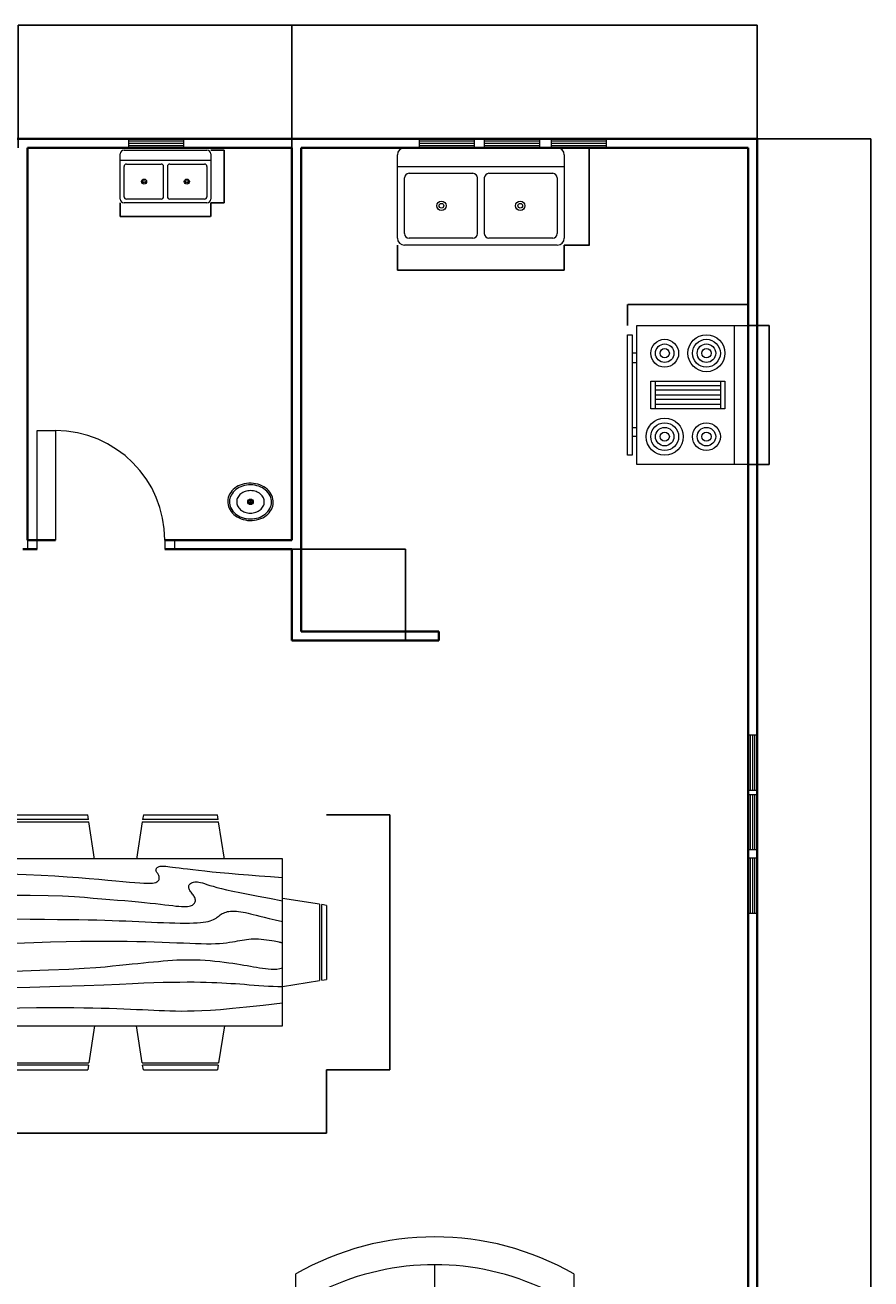
# Model space of a CAD drawing. Units: millimetres. Extents: x 1194 to 22780, y 83 to 13378.
# Tile 3 of 6: x 6855 to 11490, y 6507 to 13378. Entities that reach past the tile are written whole.
import ezdxf

# ---------------------------------------------------------------- set-up
doc = ezdxf.new("R2010")
doc.units = ezdxf.units.MM
for name, color, linetype, lineweight in [('A-ANNO-DIMS', 2, 'Continuous', 18), ('A-DOOR', 3, 'Continuous', 18), ('A-EQPM', 9, 'Continuous', 18), ('A-FLOR-FIXT', 9, 'Continuous', 18), ('A-FURN', 8, 'Continuous', 18), ('A-GLAZ', 4, 'Continuous', 18), ('A-WALL', 7, 'Continuous', 35)]:
    doc.layers.add(name, color=color, linetype=linetype, lineweight=lineweight)
doc.styles.get("Standard").update_dxf_attribs({"font": 'arial.ttf'})
doc.dimstyles.get("Standard").update_dxf_attribs({"dimtxt": 0.18, "dimasz": 0.18, "dimexe": 0.18, "dimexo": 0.0625, "dimgap": 0.09, "dimtad": 0, "dimtih": 1, "dimtoh": 1, "dimdec": 4, "dimzin": 0, "dimdsep": 46, "dimtxsty": 'Standard', "dimcen": 0.09, "dimadec": 0, "dimazin": 0, "dimtfac": 1, "dimtdec": 4, "dimtofl": 0, "dimtmove": 0, "dimatfit": 3, "dimfxl": 1, "dimtolj": 1, "dimtzin": 0, "dimarcsym": 0})

# ---------------------------------------------------------------- blocks, each defined once
blk = doc.blocks.new('Sofa - Roundback Loveseat 5 ft.')
for p, q in [((0, -32.44198), (0, -5.99998)), ((-24, -33.99998), (-24, -11.46958)), ((-23.9998, -13.38178), (23.99986, -13.38178)), ((24.00004, -33.99998), (24.00004, -11.46958)), ((-24, -32.44198), (24.00004, -32.44198))]:
    blk.add_line(p, q)
for points in [[(-24, -33.99998), (-30, -33.99998), (-30, -7.99998)], [(30.00004, -7.99998), (30.00004, -33.99998), (24.00004, -33.99998)]]:
    blk.add_lwpolyline(points)
for centre, radius, start, end in [((0, -60.24998), 60.24998, 60.13715, 119.8628), ((0, -61.38438), 55.38444, 64.32083, 115.6792)]:
    blk.add_arc(centre, radius, start, end)
blk = doc.blocks.new('Dining Set - 36 x 72 in.')
for p, q in [((-22, 27.5), (-22.1562, 26.50042)), ((-22, 27.5), (-6, 27.5)), ((-5.8437, 26.49966), (-6, 27.5)), ((6, 27.5), (5.8438, 26.50042)), ((6, 27.5), (22, 27.5)), ((22.1563, 26.49966), (22, 27.5)), ((-22.2343, 26.00059), (-23.4847, 17.99762)), ((-22.2304, 26), (-5.7608, 26)), ((-5.8416, 26.5), (-22.1534, 26.5)), ((-4.5152, 17.99762), (-5.7655, 25.99926)), ((5.7657, 26.00059), (4.5153, 17.99762)), ((5.7696, 26), (22.2392, 26)), ((22.1584, 26.5), (5.8466, 26.5)), ((23.4848, 17.99762), (22.2345, 25.99926)), ((36, 18), (-36, 18)), ((-36, 18), (-36, -18)), ((36, -18), (36, 18)), ((-45.5, 8), (-44.5004, 8.15617)), ((-44.5, -8.15843), (-44.5, 8.15338)), ((-44.0006, 8.23428), (-35.9976, 9.48474)), ((-44, 8.23041), (-44, -8.23915)), ((44.0006, 8.23428), (35.9976, 9.48474)), ((44, 8.23041), (44, -8.23915)), ((44.5, -8.15843), (44.5, 8.15338)), ((45.5, 8), (44.5005, 8.15617)), ((-45.5, 8), (-45.5, -8)), ((45.5, 8), (45.5, -8)), ((-44.4997, -8.15631), (-45.5, -8)), ((44.4997, -8.15631), (45.5, -8)), ((-35.9976, -9.48476), (-43.9993, -8.2345)), ((35.9976, -9.48476), (43.9993, -8.2345)), ((-36, -18), (36, -18)), ((-22.2343, -26.0006), (-23.4847, -17.99762)), ((-4.5152, -17.99762), (-5.7655, -25.99928)), ((5.7657, -26.0006), (4.5153, -17.99762)), ((23.4848, -17.99762), (22.2345, -25.99928)), ((-22.2304, -26), (-5.7608, -26)), ((-22, -27.5), (-22.1562, -26.50044)), ((-5.8416, -26.5), (-22.1534, -26.5)), ((-5.8437, -26.49967), (-6, -27.5)), ((5.7696, -26), (22.2392, -26)), ((6, -27.5), (5.8438, -26.50044)), ((22.1584, -26.5), (5.8466, -26.5)), ((22.1563, -26.49967), (22, -27.5)), ((-22, -27.5), (-6, -27.5)), ((6, -27.5), (22, -27.5))]:
    blk.add_line(p, q)
for points in [[(-36, 15), (-31.1772, 14.97754), (-26.8079, 14.91406), (-22.8538, 14.81543), (-19.276, 14.6875), (-16.0362, 14.53613), (-13.0957, 14.36718), (-10.4159, 14.18652), (-7.9583, 14), (-5.6904, 13.81315), (-3.6035, 13.63021), (-1.6954, 13.45508), (0.0365, 13.29166), (1.5945, 13.14388), (2.9811, 13.01562), (4.1988, 12.9108), (5.25, 12.83333), (6.1393, 12.78613), (6.8802, 12.76823), (7.4883, 12.77767), (7.9792, 12.8125), (8.3685, 12.87077), (8.6719, 12.95052), (8.9049, 13.0498), (9.0833, 13.16666), (9.2205, 13.29899), (9.3216, 13.44401), (9.3895, 13.59879), (9.4271, 13.76041), (9.4373, 13.92594), (9.4232, 14.09245), (9.3875, 14.257), (9.3333, 14.41666), (9.2638, 14.56917), (9.1836, 14.71484), (9.0975, 14.85465), (9.0104, 14.98958), (8.9272, 15.1206), (8.8529, 15.2487), (8.7922, 15.37483), (8.75, 15.5), (8.7305, 15.62467), (8.7344, 15.74739), (8.7617, 15.86621), (8.8125, 15.97916), (8.8867, 16.08431), (8.9844, 16.17968), (9.1055, 16.26334), (9.25, 16.33333), (9.4189, 16.38802), (9.6172, 16.42708), (9.8506, 16.45052), (10.125, 16.45833), (10.4463, 16.45052), (10.8203, 16.42708), (11.2529, 16.38802), (11.75, 16.33333), (12.3184, 16.26318), (12.9694, 16.17838), (13.7151, 16.07991), (14.5677, 15.96875), (15.5395, 15.84586), (16.6426, 15.71224), (17.8893, 15.56884), (19.2917, 15.41666), (20.859, 15.25667), (22.5879, 15.08984), (24.4721, 14.91715), (26.5052, 14.73958), (28.6809, 14.5581), (30.9929, 14.3737), (33.4347, 14.18733), (36, 14)], [(-36, 10), (-28.9766, 10.14274), (-23.1725, 10.20442), (-18.4241, 10.19775), (-14.5677, 10.13541), (-11.4399, 10.03011), (-8.877, 9.89453), (-6.7154, 9.74137), (-4.7917, 9.58333), (-2.9698, 9.43082), (-1.2246, 9.28515), (0.4415, 9.14534), (2.026, 9.01041), (3.5266, 8.87939), (4.9408, 8.7513), (6.266, 8.62516), (7.5, 8.5), (8.6411, 8.37549), (9.6914, 8.2539), (10.6538, 8.13818), (11.5312, 8.03125), (12.3267, 7.93603), (13.043, 7.85547), (13.6831, 7.79248), (14.25, 7.75), (14.7471, 7.7303), (15.1797, 7.73307), (15.5537, 7.75732), (15.875, 7.80208), (16.1494, 7.86637), (16.3828, 7.94922), (16.5811, 8.04964), (16.75, 8.16666), (16.8944, 8.29915), (17.0143, 8.44531), (17.1089, 8.60319), (17.1771, 8.77083), (17.218, 8.94629), (17.2305, 9.1276), (17.2137, 9.31282), (17.1667, 9.5), (17.0895, 9.6875), (16.987, 9.875), (16.8649, 10.0625), (16.7292, 10.25), (16.5856, 10.4375), (16.4401, 10.625), (16.2985, 10.8125), (16.1667, 11), (16.05, 11.18733), (15.9518, 11.3737), (15.8752, 11.5581), (15.8229, 11.73958), (15.798, 11.91715), (15.8034, 12.08984), (15.842, 12.25667), (15.9167, 12.41666), (16.0295, 12.56836), (16.1784, 12.70833), (16.3605, 12.83268), (16.5729, 12.9375), (16.8127, 13.01888), (17.0768, 13.07291), (17.3625, 13.0957), (17.6667, 13.08333), (17.9894, 13.03312), (18.3418, 12.94726), (18.7382, 12.82918), (19.1927, 12.68229), (19.7195, 12.51001), (20.3327, 12.31575), (21.0465, 12.10294), (21.875, 11.875), (22.8357, 11.63354), (23.959, 11.37304), (25.2786, 11.08618), (26.8282, 10.76562), (28.6414, 10.40405), (30.752, 9.99414), (33.1936, 9.52856), (36, 9)], [(-36, 5.5), (-30.7157, 5.3348), (-26.069, 5.20963), (-21.9946, 5.11767), (-18.4271, 5.05208), (-15.3009, 5.00602), (-12.5508, 4.97265), (-10.1112, 4.94515), (-7.9167, 4.91666), (-5.909, 4.88167), (-4.0586, 4.83984), (-2.3429, 4.79215), (-0.7396, 4.73958), (0.7739, 4.6831), (2.22, 4.6237), (3.6213, 4.56233), (5, 4.5), (6.373, 4.43782), (7.7344, 4.3776), (9.0723, 4.32129), (10.375, 4.27083), (11.6309, 4.22819), (12.8281, 4.19531), (13.9551, 4.17415), (15, 4.16666), (15.954, 4.17448), (16.819, 4.19791), (17.6001, 4.23698), (18.3021, 4.29166), (18.9299, 4.36198), (19.4883, 4.44791), (19.9823, 4.54948), (20.4167, 4.66666), (20.7969, 4.79899), (21.1302, 4.94401), (21.4245, 5.09879), (21.6875, 5.26041), (21.9271, 5.42594), (22.1511, 5.59245), (22.3672, 5.757), (22.5834, 5.91666), (22.8065, 6.06868), (23.0404, 6.21093), (23.2879, 6.34147), (23.5521, 6.45833), (23.8358, 6.55957), (24.142, 6.64323), (24.4735, 6.70735), (24.8334, 6.75), (25.2235, 6.76969), (25.642, 6.76692), (26.0858, 6.74267), (26.5521, 6.69791), (27.0379, 6.63362), (27.5404, 6.55078), (28.0565, 6.45036), (28.5834, 6.33333), (29.1242, 6.19987), (29.7071, 6.04687), (30.3661, 5.87044), (31.1354, 5.66666), (32.0493, 5.43164), (33.142, 5.16146), (34.4475, 4.85221), (36, 4.5)], [(-36, -1), (-30.7915, -0.6591), (-26.0195, -0.38216), (-21.6519, -0.16284), (-17.6563, 0.00521), (-14.0005, 0.12833), (-10.6523, 0.21289), (-7.5796, 0.26522), (-4.75, 0.29166), (-2.134, 0.29793), (0.2878, 0.28711), (2.5317, 0.26163), (4.6146, 0.22396), (6.5529, 0.17651), (8.3633, 0.12174), (10.0623, 0.06209), (11.6667, 0), (13.1899, -0.06201), (14.6341, -0.1211), (15.9982, -0.17432), (17.2813, -0.21875), (18.4823, -0.25147), (19.6003, -0.26953), (20.6343, -0.27002), (21.5834, -0.25), (22.4481, -0.20768), (23.2357, -0.14584), (23.9549, -0.06836), (24.6146, 0.02083), (25.2235, 0.11784), (25.7904, 0.21875), (26.3241, 0.31966), (26.8334, 0.41666), (27.3265, 0.50618), (27.8099, 0.58593), (28.2894, 0.65397), (28.7709, 0.70833), (29.2601, 0.74707), (29.763, 0.76823), (30.2855, 0.76985), (30.8334, 0.75), (31.4088, 0.70784), (31.9994, 0.64713), (32.589, 0.57275), (33.1615, 0.48958), (33.7008, 0.4025), (34.1908, 0.3164), (34.6153, 0.23616), (34.9584, 0.16666), (35.2099, 0.11165), (35.3848, 0.07031), (35.504, 0.04069), (35.5886, 0.02083), (35.6594, 0.00879), (35.7377, 0.0026), (35.8442, 0.00032), (36, 0)], [(-36, -6.5), (-27.1843, -6.31267), (-20.084, -6.1263), (-14.469, -5.9419), (-10.1094, -5.76042), (-6.7752, -5.58285), (-4.2363, -5.41016), (-2.2629, -5.24333), (-0.625, -5.08334), (0.8708, -4.93099), (2.2715, -4.78646), (3.5872, -4.64974), (4.8281, -4.52084), (6.0046, -4.39974), (7.127, -4.28646), (8.2053, -4.18099), (9.25, -4.08334), (10.2705, -3.99382), (11.2734, -3.91407), (12.2647, -3.84603), (13.25, -3.79167), (14.2354, -3.75293), (15.2266, -3.73177), (16.2295, -3.73015), (17.25, -3.75), (18.2912, -3.79248), (19.3451, -3.85547), (20.4009, -3.93604), (21.4479, -4.03125), (22.4754, -4.13819), (23.4727, -4.25391), (24.4289, -4.37549), (25.3334, -4.5), (26.1785, -4.62492), (26.9694, -4.74935), (27.7145, -4.87281), (28.4219, -4.99479), (29.1, -5.11483), (29.7572, -5.23242), (30.4016, -5.34709), (31.0417, -5.45834), (31.6837, -5.56437), (32.3262, -5.65821), (32.9658, -5.73153), (33.599, -5.77604), (34.2224, -5.78345), (34.8327, -5.74545), (35.4264, -5.65373), (36, -5.5)], [(-36, -10), (-26.4022, -9.81299), (-18.4675, -9.62891), (-11.9839, -9.45069), (-6.7396, -9.28125), (-2.5226, -9.12354), (0.8789, -8.98047), (3.6769, -8.85498), (6.0833, -8.75), (8.2767, -8.66765), (10.3021, -8.60677), (12.1712, -8.56543), (13.8958, -8.54167), (15.4876, -8.53353), (16.9583, -8.53907), (18.3197, -8.55632), (19.5834, -8.58334), (20.7616, -8.61841), (21.8685, -8.66081), (22.9188, -8.71004), (23.9271, -8.76563), (24.9081, -8.82707), (25.8763, -8.89388), (26.8465, -8.96558), (27.8334, -9.04167), (28.8474, -9.12118), (29.8828, -9.20117), (30.93, -9.27824), (31.9792, -9.34896), (33.0205, -9.40991), (34.0443, -9.45768), (35.0407, -9.48885), (36, -9.5)], [(-36, -14.5), (-30.0881, -14.33513), (-25.0332, -14.21224), (-20.7312, -14.12647), (-17.0781, -14.07292), (-13.97, -14.04671), (-11.3027, -14.04297), (-8.9724, -14.05681), (-6.875, -14.08334), (-4.9224, -14.11833), (-3.0905, -14.16016), (-1.3709, -14.20785), (0.2448, -14.26042), (1.7647, -14.3169), (3.1973, -14.3763), (4.5507, -14.43767), (5.8333, -14.5), (7.0554, -14.5621), (8.235, -14.62175), (9.3922, -14.67652), (10.5469, -14.72396), (11.7192, -14.76164), (12.929, -14.78711), (14.1965, -14.79794), (15.5417, -14.79167), (16.9933, -14.76424), (18.6152, -14.70508), (20.4804, -14.60197), (22.6615, -14.44271), (25.2312, -14.21509), (28.2624, -13.9069), (31.8277, -13.50594), (36, -13)]]:
    blk.add_lwpolyline(points)
blk = doc.blocks.new('Range-Oven - 30 in top')
for p, q in [((0, -3), (30, -3)), ((12, -6), (18, -6)), ((13, -20), (13, -6)), ((14, -6), (14, -20)), ((15, -20), (15, -6)), ((16, -6), (16, -20)), ((17, -20), (17, -6)), ((18, -20), (12, -20)), ((6, -24), (6, -25)), ((8, -25), (8, -24)), ((22, -25), (22, -24)), ((24, -24), (24, -25))]:
    blk.add_line(p, q)
for points in [[(0, -24), (0, 0), (30, 0), (30, -24)], [(12, -21), (12, -5), (18, -5), (18, -21)], [(2, -26), (2, -25), (28, -25), (28, -26)]]:
    blk.add_lwpolyline(points, close=True)
for centre, radius in [((6, -9), 4), ((6, -9), 3), ((6, -9), 2), ((6, -9), 1), ((24, -9), 3), ((24, -9), 2), ((24, -9), 1), ((6, -18), 3), ((6, -18), 2), ((24, -18), 4), ((24, -18), 3), ((24, -18), 2), ((6, -18), 1), ((24, -18), 1)]:
    blk.add_circle(centre, radius)
blk = doc.blocks.new('Sink-double - 36 in top')
for p, q in [((-18, -4), (18, -4)), ((-0.75, -18.5), (-0.75, -6.5)), ((0.75, -6.5), (0.75, -18.5))]:
    blk.add_line(p, q)
for points in [[(-16.5, 0), (16.5, 0)], [(-18, -19.5), (-18, -1.5)], [(18, -1.5), (18, -19.5)], [(-16.5, -18.5), (-16.5, -6.5)], [(-15.5, -5.5), (-1.75, -5.5)], [(1.75, -5.5), (15.5, -5.5)], [(16.5, -6.5), (16.5, -18.5)], [(16.5, -21), (-16.5, -21)], [(-1.75, -19.5), (-15.5, -19.5)], [(15.5, -19.5), (1.75, -19.5)]]:
    blk.add_lwpolyline(points)
for centre, radius in [((-8.5, -12.5), 1), ((-8.5, -12.5), 0.5), ((8.5, -12.5), 1), ((8.5, -12.5), 0.5)]:
    blk.add_circle(centre, radius)
for centre, radius, start, end in [((-16.5, -1.5), 1.5, 90, 180), ((16.5, -1.5), 1.5, 0, 90), ((-15.5, -6.5), 1, 90, 180), ((-1.75, -6.5), 1, 0, 90), ((1.75, -6.5), 1, 90, 180), ((15.5, -6.5), 1, 0, 90), ((-15.5, -18.5), 1, 180, 270), ((-1.75, -18.5), 1, 270, 0), ((1.75, -18.5), 1, 180, 270), ((15.5, -18.5), 1, 270, 0), ((-16.5, -19.5), 1.5, 180, 270), ((16.5, -19.5), 1.5, 270, 0)]:
    blk.add_arc(centre, radius, start, end)
blk = doc.blocks.new('Sink - Oval top')
for p, q in [((-1, 0), (1, 0)), ((0, 1), (0, -1))]:
    blk.add_line(p, q)
for points in [[(-12.23, 0.39, 0.117634), (-11.46, -3.36, 0.104469), (-8.88, -6.8, 0.090016), (-5.08, -9.07, 0.08192), (-0.32, -10.02, 0.08192), (4.49, -9.38, 0.090016), (8.42, -7.36, 0.104469), (11.22, -4.09, 0.117634), (12.23, -0.39, 0.117634), (11.46, 3.36, 0.104469), (8.88, 6.8, 0.090016), (5.08, 9.07, 0.08192), (0.32, 10.02, 0.08192), (-4.49, 9.38, 0.090016), (-8.42, 7.36, 0.104469), (-11.22, 4.09, 0.117634)], [(-11.29, 0.16, 0.118622), (-10.52, -3.25, 0.104678), (-8.07, -6.36, 0.089562), (-4.54, -8.37, 0.081185), (-0.13, -9.15, 0.081185), (4.3, -8.49, 0.089562), (7.89, -6.58, 0.104678), (10.42, -3.55, 0.118622), (11.29, -0.16, 0.118622), (10.52, 3.25, 0.104678), (8.07, 6.36, 0.089562), (4.54, 8.37, 0.081185), (0.13, 9.15, 0.081185), (-4.3, 8.49, 0.089562), (-7.89, 6.58, 0.104678), (-10.42, 3.55, 0.118622)], [(-7.42, 0.08, 0.118283), (-6.91, -2.17, 0.104607), (-5.29, -4.21, 0.089718), (-2.97, -5.53, 0.081436), (-0.07, -6.04, 0.081436), (2.84, -5.59, 0.089718), (5.2, -4.33, 0.104607), (6.86, -2.32, 0.118283), (7.42, -0.08, 0.118283), (6.91, 2.17, 0.104607), (5.29, 4.21, 0.089718), (2.97, 5.53, 0.081436), (0.07, 6.04, 0.081436), (-2.84, 5.59, 0.089718), (-5.2, 4.33, 0.104607), (-6.86, 2.32, 0.118283)]]:
    blk.add_lwpolyline(points, format="xyb", close=True)
for radius in [1.5, 1]:
    blk.add_circle((0, 0), radius)
blk = doc.blocks.new('Window - Wood Frame 36 in. Wide plan')
for p, q in [((0, 6), (0, 0)), ((0, 4.5), (36, 4.5)), ((0, 3), (36, 3)), ((0, 1.5), (36, 1.5)), ((36, 6), (36, 0))]:
    blk.add_line(p, q)
blk = doc.blocks.new('DOOR-SWING-600')
for p, q in [((0, 0), (0, 600)), ((0, 600), (100, 600)), ((100, 600), (100, 0))]:
    blk.add_line(p, q)
blk.add_arc((100, 0), 600, 0, 90)
blk = doc.blocks.new('*D35')
at = {"layer": 'A-ANNO-DIMS', "color": 0, "lineweight": -2, "transparency": 16777216}
for p, q in [((8895.5, 12172.3), (8895.5, 12035)), ((9809.9, 12172.3), (9809.9, 12035)), ((8895.7, 12035.2), (9352.1, 12035.2)), ((9809.7, 12035.2), (9353.3, 12035.2))]:
    blk.add_line(p, q, dxfattribs=at)
at = {"layer": 'A-ANNO-DIMS', "color": 0, "transparency": 16777216}
for points in [[(8895.7, 12035.2), (8895.7, 12035.2), (8895.5, 12035.2)], [(9809.7, 12035.2), (9809.7, 12035.2), (9809.9, 12035.2)]]:
    blk.add_solid(points, dxfattribs=at)
at = {"layer": 'Defpoints', "color": 0, "transparency": 16777216}
for p in [(8895.5, 12172.4), (9809.9, 12172.4), (9809.9, 12035.2)]:
    blk.add_point(p, dxfattribs=at)
at = {"layer": 'A-ANNO-DIMS', "color": 0, "transparency": 16777216, "insert": (9352.7, 12035.2), "char_height": 0.18, "attachment_point": 5}
blk.add_mtext('\\A1;SINK 914', dxfattribs=at)
blk = doc.blocks.new('*D36')
at = {"layer": 'A-ANNO-DIMS', "color": 0, "lineweight": -2, "transparency": 16777216}
for p, q in [((9810, 12705.8), (9947.2, 12705.8)), ((9947.1, 12705.6), (9947.1, 12439.3)), ((9947.1, 12172.6), (9947.1, 12438.9)), ((9810, 12172.4), (9947.2, 12172.4))]:
    blk.add_line(p, q, dxfattribs=at)
at = {"layer": 'A-ANNO-DIMS', "color": 0, "transparency": 16777216}
for points in [[(9947, 12705.6), (9947.1, 12705.6), (9947.1, 12705.8)], [(9947, 12172.6), (9947.1, 12172.6), (9947.1, 12172.4)]]:
    blk.add_solid(points, dxfattribs=at)
at = {"layer": 'Defpoints', "color": 0, "transparency": 16777216}
for p in [(9809.9, 12705.8), (9947.1, 12705.8), (9809.9, 12172.4)]:
    blk.add_point(p, dxfattribs=at)
at = {"layer": 'A-ANNO-DIMS', "color": 0, "transparency": 16777216, "insert": (9947.1, 12439.1), "char_height": 0.18, "attachment_point": 5}
blk.add_mtext('\\A1;533', dxfattribs=at)
blk = doc.blocks.new('*D37')
at = {"layer": 'A-ANNO-DIMS', "color": 0, "lineweight": -2, "transparency": 16777216}
for p, q in [((7376.4, 12403.6), (7376.4, 12329.1)), ((7872.2, 12403.6), (7872.2, 12329.1)), ((7376.6, 12329.3), (7623.7, 12329.3)), ((7872, 12329.3), (7624.9, 12329.3))]:
    blk.add_line(p, q, dxfattribs=at)
at = {"layer": 'A-ANNO-DIMS', "color": 0, "transparency": 16777216}
for points in [[(7376.6, 12329.3), (7376.6, 12329.3), (7376.4, 12329.3)], [(7872, 12329.3), (7872, 12329.3), (7872.2, 12329.3)]]:
    blk.add_solid(points, dxfattribs=at)
at = {"layer": 'Defpoints', "color": 0, "transparency": 16777216}
for p in [(7376.4, 12403.7), (7872.2, 12403.7), (7872.2, 12329.3)]:
    blk.add_point(p, dxfattribs=at)
at = {"layer": 'A-ANNO-DIMS', "color": 0, "transparency": 16777216, "insert": (7624.3, 12329.3), "char_height": 0.18, "attachment_point": 5}
blk.add_mtext('\\A1;SINK 496', dxfattribs=at)
blk = doc.blocks.new('*D38')
at = {"layer": 'A-ANNO-DIMS', "color": 0, "lineweight": -2, "transparency": 16777216}
for p, q in [((7872.2, 12692.8), (7946.7, 12692.8)), ((7946.5, 12692.7), (7946.5, 12548.4)), ((7946.5, 12403.8), (7946.5, 12548.1)), ((7872.2, 12403.7), (7946.7, 12403.7))]:
    blk.add_line(p, q, dxfattribs=at)
at = {"layer": 'A-ANNO-DIMS', "color": 0, "transparency": 16777216}
for points in [[(7946.5, 12692.7), (7946.6, 12692.7), (7946.5, 12692.8)], [(7946.5, 12403.8), (7946.6, 12403.8), (7946.5, 12403.7)]]:
    blk.add_solid(points, dxfattribs=at)
at = {"layer": 'Defpoints', "color": 0, "transparency": 16777216}
for p in [(7872.2, 12692.8), (7946.5, 12692.8), (7872.2, 12403.7)]:
    blk.add_point(p, dxfattribs=at)
at = {"layer": 'A-ANNO-DIMS', "color": 0, "transparency": 16777216, "insert": (7946.5, 12548.2), "char_height": 0.18, "attachment_point": 5}
blk.add_mtext('\\A1;289', dxfattribs=at)
blk = doc.blocks.new('*D45')
at = {"layer": 'A-ANNO-DIMS', "color": 0, "lineweight": -2, "transparency": 16777216}
for p, q in [((6195, 7652.6), (6195, 7305.8)), ((8506.4, 7652.6), (8506.4, 7305.8)), ((6195.2, 7306), (7349.6, 7306)), ((8506.2, 7306), (7351.8, 7306))]:
    blk.add_line(p, q, dxfattribs=at)
at = {"layer": 'A-ANNO-DIMS', "color": 0, "transparency": 16777216}
for points in [[(6195.2, 7306), (6195.2, 7305.9), (6195, 7306)], [(8506.2, 7306), (8506.2, 7305.9), (8506.4, 7306)]]:
    blk.add_solid(points, dxfattribs=at)
at = {"layer": 'Defpoints', "color": 0, "transparency": 16777216}
for p in [(6195, 7652.7), (8506.4, 7652.7), (8506.4, 7306)]:
    blk.add_point(p, dxfattribs=at)
at = {"layer": 'A-ANNO-DIMS', "color": 0, "transparency": 16777216, "insert": (7350.7, 7306), "char_height": 0.18, "attachment_point": 5}
blk.add_mtext('\\A1;DINING SET 2311', dxfattribs=at)
blk = doc.blocks.new('*D46')
at = {"layer": 'A-ANNO-DIMS', "color": 0, "lineweight": -2, "transparency": 16777216}
for p, q in [((8506.4, 9049.7), (8853.3, 9049.7)), ((8853.1, 9049.5), (8853.1, 8351.4)), ((8853.1, 7652.8), (8853.1, 8351)), ((8506.4, 7652.7), (8853.3, 7652.7))]:
    blk.add_line(p, q, dxfattribs=at)
at = {"layer": 'A-ANNO-DIMS', "color": 0, "transparency": 16777216}
for points in [[(8853.1, 9049.5), (8853.1, 9049.5), (8853.1, 9049.7)], [(8853.1, 7652.8), (8853.1, 7652.8), (8853.1, 7652.7)]]:
    blk.add_solid(points, dxfattribs=at)
at = {"layer": 'Defpoints', "color": 0, "transparency": 16777216}
for p in [(8506.4, 9049.7), (8853.1, 9049.7), (8506.4, 7652.7)]:
    blk.add_point(p, dxfattribs=at)
at = {"layer": 'A-ANNO-DIMS', "color": 0, "transparency": 16777216, "insert": (8853.1, 8351.2), "char_height": 0.18, "attachment_point": 5}
blk.add_mtext('\\A1;1397', dxfattribs=at)
blk = doc.blocks.new('*D47')
at = {"layer": 'A-ANNO-DIMS', "color": 0, "lineweight": -2, "transparency": 16777216}
for p, q in [((10817.5, 11732.6), (10932, 11732.6)), ((10931.8, 11732.4), (10931.8, 11351.8)), ((10931.8, 10970.8), (10931.8, 11351.4)), ((10817.5, 10970.6), (10932, 10970.6))]:
    blk.add_line(p, q, dxfattribs=at)
at = {"layer": 'A-ANNO-DIMS', "color": 0, "transparency": 16777216}
for points in [[(10931.8, 11732.4), (10931.8, 11732.4), (10931.8, 11732.6)], [(10931.8, 10970.8), (10931.8, 10970.8), (10931.8, 10970.6)]]:
    blk.add_solid(points, dxfattribs=at)
at = {"layer": 'Defpoints', "color": 0, "transparency": 16777216}
for p in [(10817.5, 11732.6), (10817.5, 10970.6), (10931.8, 10970.6)]:
    blk.add_point(p, dxfattribs=at)
at = {"layer": 'A-ANNO-DIMS', "color": 0, "transparency": 16777216, "insert": (10931.8, 11351.6), "char_height": 0.18, "attachment_point": 5}
blk.add_mtext('\\A1;RANGE 762', dxfattribs=at)
blk = doc.blocks.new('*D48')
at = {"layer": 'A-ANNO-DIMS', "color": 0, "lineweight": -2, "transparency": 16777216}
for p, q in [((10157.1, 11732.7), (10157.1, 11847.1)), ((10157.3, 11846.9), (10487, 11846.9)), ((10817.3, 11846.9), (10487.6, 11846.9)), ((10817.5, 11732.7), (10817.5, 11847.1))]:
    blk.add_line(p, q, dxfattribs=at)
at = {"layer": 'A-ANNO-DIMS', "color": 0, "transparency": 16777216}
for points in [[(10157.3, 11846.9), (10157.3, 11846.9), (10157.1, 11846.9)], [(10817.3, 11846.9), (10817.3, 11846.9), (10817.5, 11846.9)]]:
    blk.add_solid(points, dxfattribs=at)
at = {"layer": 'Defpoints', "color": 0, "transparency": 16777216}
for p in [(10817.5, 11846.9), (10157.1, 11732.6), (10817.5, 11732.6)]:
    blk.add_point(p, dxfattribs=at)
at = {"layer": 'A-ANNO-DIMS', "color": 0, "transparency": 16777216, "insert": (10487.3, 11846.9), "char_height": 0.18, "attachment_point": 5}
blk.add_mtext('\\A1;660', dxfattribs=at)
blk = doc.blocks.new('*D52')
at = {"layer": 'A-ANNO-DIMS', "color": 0, "lineweight": -2, "transparency": 16777216}
for p, q in [((10867.5, 12755.8), (11490.2, 12755.8)), ((11490, 12755.6), (11490, 6731)), ((11490, 706), (11490, 6730.6)), ((10867.5, 705.8), (11490.2, 705.8))]:
    blk.add_line(p, q, dxfattribs=at)
at = {"layer": 'A-ANNO-DIMS', "color": 0, "transparency": 16777216}
for points in [[(11490, 12755.6), (11490, 12755.6), (11490, 12755.8)], [(11490, 706), (11490, 706), (11490, 705.8)]]:
    blk.add_solid(points, dxfattribs=at)
at = {"layer": 'Defpoints', "color": 0, "transparency": 16777216}
for p in [(10867.5, 12755.8), (11490, 12755.8), (10867.5, 705.8)]:
    blk.add_point(p, dxfattribs=at)
at = {"layer": 'A-ANNO-DIMS', "color": 0, "transparency": 16777216, "insert": (11490, 6730.8), "char_height": 0.18, "attachment_point": 5}
blk.add_mtext('\\A1;12050', dxfattribs=at)
blk = doc.blocks.new('*D55')
at = {"layer": 'A-ANNO-DIMS', "color": 0, "lineweight": -2, "transparency": 16777216}
for p, q in [((6817.5, 12705.8), (6817.5, 13378.5)), ((6817.7, 13378.3), (7567.1, 13378.3)), ((8317.3, 13378.3), (7567.8, 13378.3)), ((8317.5, 12705.8), (8317.5, 13378.5))]:
    blk.add_line(p, q, dxfattribs=at)
at = {"layer": 'A-ANNO-DIMS', "color": 0, "transparency": 16777216}
for points in [[(6817.7, 13378.3), (6817.7, 13378.2), (6817.5, 13378.3)], [(8317.3, 13378.3), (8317.3, 13378.2), (8317.5, 13378.3)]]:
    blk.add_solid(points, dxfattribs=at)
at = {"layer": 'Defpoints', "color": 0, "transparency": 16777216}
for p in [(8317.5, 13378.3), (6817.5, 12705.8), (8317.5, 12705.8)]:
    blk.add_point(p, dxfattribs=at)
at = {"layer": 'A-ANNO-DIMS', "color": 0, "transparency": 16777216, "insert": (7567.5, 13378.3), "char_height": 0.18, "attachment_point": 5}
blk.add_mtext('\\A1;1500', dxfattribs=at)
blk = doc.blocks.new('*D56')
at = {"layer": 'A-ANNO-DIMS', "color": 0, "lineweight": -2, "transparency": 16777216}
for p, q in [((8317.4811, 12705.836385), (8317.4811, 13378.453885)), ((8317.6611, 13378.273885), (9592.1211, 13378.273885)), ((10867.3011, 13378.273885), (9592.8411, 13378.273885)), ((10867.4811, 12755.836385), (10867.4811, 13378.453885))]:
    blk.add_line(p, q, dxfattribs=at)
at = {"layer": 'A-ANNO-DIMS', "color": 0, "transparency": 16777216}
for points in [[(8317.6611, 13378.303885), (8317.6611, 13378.243885), (8317.4811, 13378.273885)], [(10867.3011, 13378.303885), (10867.3011, 13378.243885), (10867.4811, 13378.273885)]]:
    blk.add_solid(points, dxfattribs=at)
at = {"layer": 'Defpoints', "color": 0, "transparency": 16777216}
for p in [(10867.4811, 13378.273885), (10867.4811, 12755.773885), (8317.4811, 12705.773885)]:
    blk.add_point(p, dxfattribs=at)
at = {"layer": 'A-ANNO-DIMS', "color": 0, "transparency": 16777216, "insert": (9592.4811, 13378.273885), "char_height": 0.18, "attachment_point": 5}
blk.add_mtext('\\A1;2550', dxfattribs=at)
blk = doc.blocks.new('*D64')
at = {"layer": 'A-ANNO-DIMS', "color": 0, "lineweight": -2, "transparency": 16777216}
for p, q in [((8317.5, 10505.8), (8940.2, 10505.8)), ((8940, 10505.6), (8940, 10256)), ((8940, 10006), (8940, 10255.6)), ((8317.5, 10005.8), (8940.2, 10005.8))]:
    blk.add_line(p, q, dxfattribs=at)
at = {"layer": 'A-ANNO-DIMS', "color": 0, "transparency": 16777216}
for points in [[(8940, 10505.6), (8940, 10505.6), (8940, 10505.8)], [(8940, 10006), (8940, 10006), (8940, 10005.8)]]:
    blk.add_solid(points, dxfattribs=at)
at = {"layer": 'Defpoints', "color": 0, "transparency": 16777216}
for p in [(8317.5, 10505.8), (8317.5, 10005.8), (8940, 10005.8)]:
    blk.add_point(p, dxfattribs=at)
at = {"layer": 'A-ANNO-DIMS', "color": 0, "transparency": 16777216, "insert": (8940, 10255.8), "char_height": 0.18, "attachment_point": 5}
blk.add_mtext('\\A1;500', dxfattribs=at)

msp = doc.modelspace()

# ---------------------------------------------------------------- linework, layer by layer
at = {"layer": 'A-DOOR'}
for p, q in [((6867.426, 10555.774), (6867.426, 10505.774)), ((6921.111, 10505.774), (6921.111, 10555.774)), ((7621.111, 10555.774), (7621.111, 10505.774)), ((7674.796, 10505.774), (7674.796, 10555.774)), ((6867.426, 10505.774), (6921.111, 10505.774)), ((7621.111, 10505.774), (7674.796, 10505.774))]:
    msp.add_line(p, q, dxfattribs=at)
at = {"layer": 'A-WALL'}
for p, q in [((10842.481, 12755.774), (1842.481, 12755.774)), ((1842.481, 12755.774), (10867.481, 12755.774)), ((10867.481, 12755.774), (10867.481, 12730.774)), ((10867.481, 730.774), (10867.481, 12730.774)), ((6867.481, 12705.774), (6867.481, 10555.774)), ((8317.481, 12705.774), (6867.481, 12705.774)), ((8317.481, 12705.774), (8317.481, 10555.774)), ((8317.481, 12705.774), (8317.481, 10555.774)), ((8367.481, 12705.774), (8367.481, 10530.774)), ((8367.481, 12705.774), (8367.481, 10055.774)), ((10817.481, 12705.774), (8367.481, 12705.774)), ((10817.481, 10055.774), (10817.481, 12705.774)), ((7021.111, 10555.774), (6867.481, 10555.774)), ((8317.481, 10555.774), (7621.111, 10555.774)), ((6921.111, 10505.774), (6842.481, 10505.774)), ((8317.481, 10505.774), (7621.111, 10505.774)), ((8317.481, 10505.774), (8317.481, 10030.774)), ((8367.481, 10055.774), (9122.003, 10055.774)), ((9122.003, 10055.774), (9122.003, 10005.774)), ((10817.481, 10055.774), (10817.481, 10005.774)), ((8317.481, 10030.774), (8317.481, 10005.774)), ((8317.481, 10005.774), (8342.481, 10005.774)), ((8342.481, 10005.774), (9122.003, 10005.774)), ((10817.481, 10005.774), (10817.481, 6930.774)), ((10817.481, 3355.774), (10817.481, 10005.774)), ((10867.481, 10030.774), (10867.481, 6930.774)), ((10817.481, 6930.774), (10817.481, 3355.774)), ((10867.481, 6930.774), (10867.481, 3330.774))]:
    msp.add_line(p, q, dxfattribs=at)

# ---------------------------------------------------------------- block references
at = {"layer": 'A-DOOR'}
msp.add_blockref('DOOR-SWING-600', (6921.111, 10555.774), dxfattribs=at)
at = {"layer": 'A-EQPM', "xscale": 25.4, "yscale": 25.4, "zscale": 25.4, "rotation": 270}
msp.add_blockref('Range-Oven - 30 in top', (10817.481, 11732.591), dxfattribs=at)
at = {"layer": 'A-FLOR-FIXT'}
for name, p, xscale, yscale, zscale in [('Sink-double - 36 in top', (7624.303, 12692.832), 13.7699985524719, 13.7699985524719, 13.7699985524719), ('Sink-double - 36 in top', (9352.7, 12705.774), 25.4, 25.4, 25.4), ('Sink - Oval top', (8090.252, 10765.506), 10.19841034025665, 10.19841034025665, 10.19841034025665)]:
    msp.add_blockref(name, p, dxfattribs=dict(at, xscale=xscale, yscale=yscale, zscale=zscale))
at = {"layer": 'A-FURN', "xscale": 25.4, "yscale": 25.4, "zscale": 25.4}
for name, p in [('Dining Set - 36 x 72 in.', (7350.673, 8351.169)), ('Sofa - Roundback Loveseat 5 ft.', (9100.23, 6737.504))]:
    msp.add_blockref(name, p, dxfattribs=at)
at = {"layer": 'A-GLAZ', "xscale": 8.388003104210137, "yscale": 8.388003104210137, "zscale": 8.388003104210137}
for p in [(7420.951, 12705.446), (9014.12, 12705.446), (9371.656, 12705.446), (9737.144, 12705.446)]:
    msp.add_blockref('Window - Wood Frame 36 in. Wide plan', p, dxfattribs=at)
at = {"layer": 'A-GLAZ', "xscale": 8.388003104210137, "yscale": 8.388003104210137, "zscale": 8.388003104210137, "rotation": 90}
for p in [(10867.481, 9186.069), (10867.481, 8860.334), (10867.481, 8512.349)]:
    msp.add_blockref('Window - Wood Frame 36 in. Wide plan', p, dxfattribs=at)

# ---------------------------------------------------------------- dimensions: what is measured, and where the dimension line sits
at = {"layer": 'A-ANNO-DIMS'}
for base, p1, p2, picture, middle in [((8317.481, 13378.274), (6817.481, 12705.774), (8317.481, 12705.774), '*D55', (7567.481, 13378.274)), ((10867.481, 13378.274), (8317.481, 12705.774), (10867.481, 12755.774), '*D56', (9592.481, 13378.274)), ((10817.481, 11846.891), (10157.081, 11732.591), (10817.481, 11732.591), '*D48', (10487.281, 11846.891))]:
    dim = msp.add_linear_dim(base=base, p1=p1, p2=p2, dimstyle='Standard', override={"dimdec": 0, "dimlfac": 1, "dimrnd": 0, "dimzin": 0, "dimdsep": 46, "dimlunit": 2}, dxfattribs=at)
    dim.commit()
    dim.dimension.update_dxf_attribs({"geometry": picture, "text_midpoint": middle})
for base, p1, p2, angle, picture, middle in [((11489.981, 12755.774), (10867.481, 705.774), (10867.481, 12755.774), 90, '*D52', (11489.981, 6730.774)), ((7946.521, 12692.832), (7872.163, 12403.662), (7872.163, 12692.832), 90, '*D38', (7946.521, 12548.247)), ((9947.06, 12705.774), (9809.9, 12172.374), (9809.9, 12705.774), 90, '*D36', (9947.06, 12439.074)), ((8939.981, 10005.774), (8317.481, 10505.774), (8317.481, 10005.774), 270, '*D64', (8939.981, 10255.774)), ((8853.083, 9049.669), (8506.373, 7652.669), (8506.373, 9049.669), 90, '*D46', (8853.083, 8351.169))]:
    dim = msp.add_linear_dim(base=base, p1=p1, p2=p2, angle=angle, dimstyle='Standard', override={"dimdec": 0, "dimlfac": 1, "dimrnd": 0, "dimzin": 0, "dimdsep": 46, "dimlunit": 2}, dxfattribs=at)
    dim.commit()
    dim.dimension.update_dxf_attribs({"geometry": picture, "text_midpoint": middle})
for base, p1, p2, text, picture, middle in [((7872.163, 12329.304), (7376.443, 12403.662), (7872.163, 12403.662), 'SINK <>', '*D37', (7624.303, 12329.304)), ((9809.9, 12035.214), (8895.5, 12172.374), (9809.9, 12172.374), 'SINK <>', '*D35', (9352.7, 12035.214)), ((8506.373, 7305.959), (6194.973, 7652.669), (8506.373, 7652.669), 'DINING SET <>', '*D45', (7350.673, 7305.959))]:
    dim = msp.add_linear_dim(base=base, p1=p1, p2=p2, text=text, dimstyle='Standard', override={"dimdec": 0, "dimlfac": 1, "dimrnd": 0, "dimzin": 0, "dimdsep": 46, "dimlunit": 2}, dxfattribs=at)
    dim.commit()
    dim.dimension.update_dxf_attribs({"geometry": picture, "text_midpoint": middle})
dim = msp.add_linear_dim(base=(10931.781, 10970.591), p1=(10817.481, 11732.591), p2=(10817.481, 10970.591), angle=270, text='RANGE <>', dimstyle='Standard', override={"dimdec": 0, "dimlfac": 1, "dimrnd": 0, "dimzin": 0, "dimdsep": 46, "dimlunit": 2}, dxfattribs=at)
dim.commit()
dim.dimension.update_dxf_attribs({"geometry": '*D47', "text_midpoint": (10931.781, 11351.591)})

doc.saveas('drawing.dxf')
